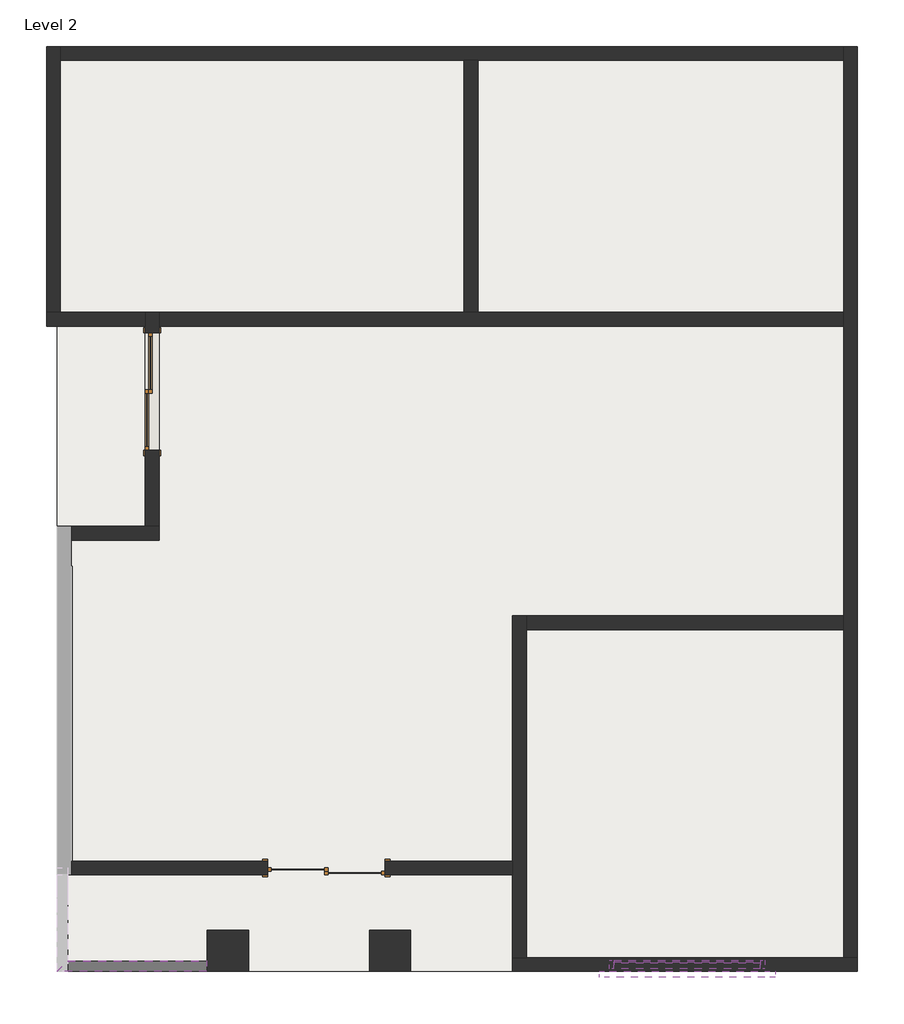
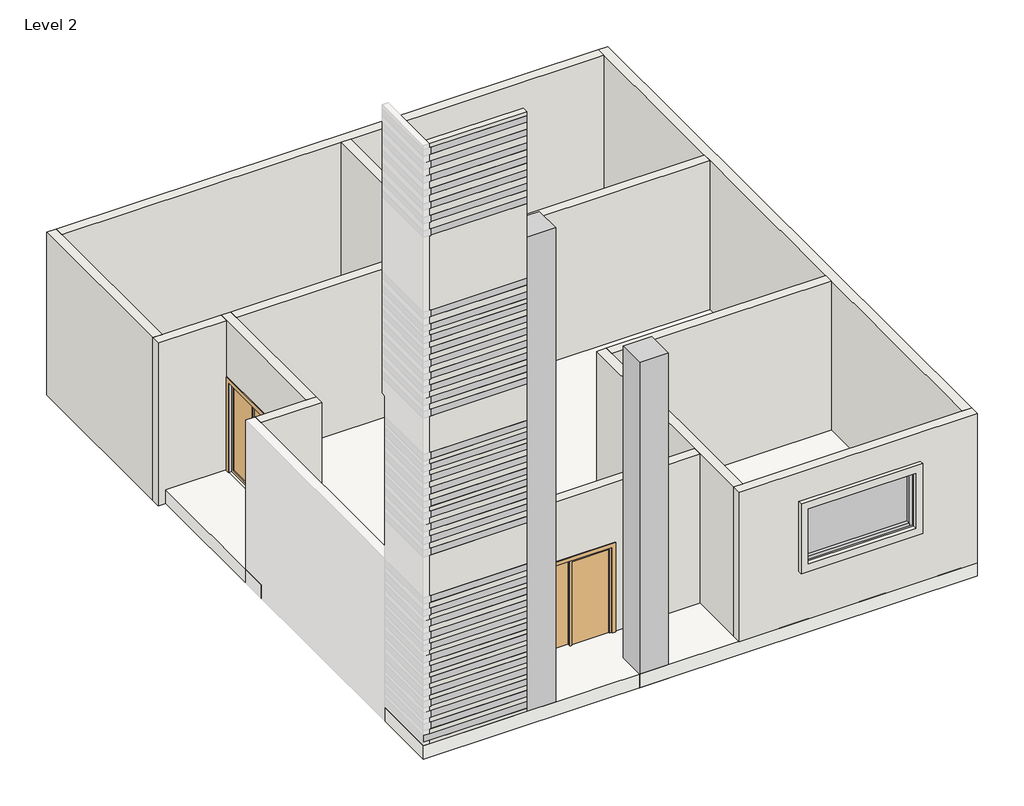
# One storey, part 2 of 2: 38 proxies, 14 walls, 8 members, 2 columns, 2 doors, 2 plates, 1 roof.
"""IFC4 building model written with IfcOpenShell, lengths in millimetres."""

from ifc_helpers import new_model, si_unit, frame, origin, place, context, project, spatial, polyline, outline, extrude, faceted_brep, transform, mapped, element, save
from components import column_feb29232, door_076b30e0, member_3a6679d5, member_c08f7e50, system_panel_glazed_5a0db22b, walls_1_walls_1_d8ce8ff7

model = new_model("IFC4")

# Units and contexts
model_context = context("Model", 3, world=origin())
ifc_project = project(units=[si_unit("LENGTHUNIT", "METRE", prefix="MILLI")], contexts=[model_context])

# Site, building, storey
site = spatial("IfcSite", under=ifc_project)
building = spatial("IfcBuilding", under=site)
storey = spatial("IfcBuildingStorey", under=building, Name="Level 2", Elevation=3657.6)

# Proxies
placement = place(None, origin())
element("IfcBuildingElementProxy", 1, Name="Reveal", ObjectType="Reveal", at=placement, inside=storey, context=model_context, shape_type="SweptSolid", body=[
    extrude(outline(polyline([(-8860.5727738, -3989.2325754), (-8708.1727738, -3836.8325754), (-6663.4727738, -3836.8325754), (-6663.4727738, -3989.2325754), (-8860.5727738, -3989.2325754)])), frame((0.0, 0.0, 4038.6), z_axis=(0.0, 0.0, 1.0), x_axis=(1.0, 0.0, 0.0)), (0.0, 0.0, 1.0), 152.4),
])
element("IfcBuildingElementProxy", 2, Name="Reveal", ObjectType="Reveal", at=placement, inside=storey, context=model_context, shape_type="SweptSolid", body=[
    extrude(outline(polyline([(-8860.5727738, -3989.2325754), (-8708.1727738, -3836.8325754), (-6663.4727738, -3836.8325754), (-6663.4727738, -3989.2325754), (-8860.5727738, -3989.2325754)])), frame((0.0, 0.0, 4292.6), z_axis=(0.0, 0.0, 1.0), x_axis=(1.0, 0.0, 0.0)), (0.0, 0.0, 1.0), 152.4),
])
element("IfcBuildingElementProxy", 3, Name="Reveal", ObjectType="Reveal", at=placement, inside=storey, context=model_context, shape_type="SweptSolid", body=[
    extrude(outline(polyline([(-8860.5727738, -3989.2325754), (-8708.1727738, -3836.8325754), (-6663.4727738, -3836.8325754), (-6663.4727738, -3989.2325754), (-8860.5727738, -3989.2325754)])), frame((0.0, 0.0, 4546.6), z_axis=(0.0, 0.0, 1.0), x_axis=(1.0, 0.0, 0.0)), (0.0, 0.0, 1.0), 152.4),
])
element("IfcBuildingElementProxy", 4, Name="Reveal", ObjectType="Reveal", at=placement, inside=storey, context=model_context, shape_type="SweptSolid", body=[
    extrude(outline(polyline([(-8860.5727738, -3989.2325754), (-8708.1727738, -3836.8325754), (-6663.4727738, -3836.8325754), (-6663.4727738, -3989.2325754), (-8860.5727738, -3989.2325754)])), frame((0.0, 0.0, 4800.6), z_axis=(0.0, 0.0, 1.0), x_axis=(1.0, 0.0, 0.0)), (0.0, 0.0, 1.0), 152.4),
])
element("IfcBuildingElementProxy", 5, Name="Reveal", ObjectType="Reveal", at=placement, inside=storey, context=model_context, shape_type="SweptSolid", body=[
    extrude(outline(polyline([(-8860.5727738, -3989.2325754), (-8708.1727738, -3836.8325754), (-6663.4727738, -3836.8325754), (-6663.4727738, -3989.2325754), (-8860.5727738, -3989.2325754)])), frame((0.0, 0.0, 5054.6), z_axis=(0.0, 0.0, 1.0), x_axis=(1.0, 0.0, 0.0)), (0.0, 0.0, 1.0), 152.4),
])
element("IfcBuildingElementProxy", 6, Name="Reveal", ObjectType="Reveal", at=placement, inside=storey, context=model_context, shape_type="SweptSolid", body=[
    extrude(outline(polyline([(-8860.5727738, -3989.2325754), (-8708.1727738, -3836.8325754), (-6663.4727738, -3836.8325754), (-6663.4727738, -3989.2325754), (-8860.5727738, -3989.2325754)])), frame((0.0, 0.0, 5308.6), z_axis=(0.0, 0.0, 1.0), x_axis=(1.0, 0.0, 0.0)), (0.0, 0.0, 1.0), 152.4),
])
element("IfcBuildingElementProxy", 7, Name="Reveal", ObjectType="Reveal", at=placement, inside=storey, context=model_context, shape_type="SweptSolid", body=[
    extrude(outline(polyline([(-8860.5727738, -3989.2325754), (-8708.1727738, -3836.8325754), (-6663.4727738, -3836.8325754), (-6663.4727738, -3989.2325754), (-8860.5727738, -3989.2325754)])), frame((0.0, 0.0, 5562.6), z_axis=(0.0, 0.0, 1.0), x_axis=(1.0, 0.0, 0.0)), (0.0, 0.0, 1.0), 152.4),
])
element("IfcBuildingElementProxy", 8, Name="Reveal", ObjectType="Reveal", at=placement, inside=storey, context=model_context, shape_type="SweptSolid", body=[
    extrude(outline(polyline([(-8860.5727738, -3989.2325754), (-8708.1727738, -3836.8325754), (-6663.4727738, -3836.8325754), (-6663.4727738, -3989.2325754), (-8860.5727738, -3989.2325754)])), frame((0.0, 0.0, 5816.6), z_axis=(0.0, 0.0, 1.0), x_axis=(1.0, 0.0, 0.0)), (0.0, 0.0, 1.0), 152.4),
])
element("IfcBuildingElementProxy", 9, Name="Reveal", ObjectType="Reveal", at=placement, inside=storey, context=model_context, shape_type="SweptSolid", body=[
    extrude(outline(polyline([(-8860.5727738, -3989.2325754), (-8708.1727738, -3836.8325754), (-6663.4727738, -3836.8325754), (-6663.4727738, -3989.2325754), (-8860.5727738, -3989.2325754)])), frame((0.0, 0.0, 6070.6), z_axis=(0.0, 0.0, 1.0), x_axis=(1.0, 0.0, 0.0)), (0.0, 0.0, 1.0), 152.4),
])
element("IfcBuildingElementProxy", 10, Name="Reveal", ObjectType="Reveal", at=placement, inside=storey, context=model_context, shape_type="SweptSolid", body=[
    extrude(outline(polyline([(-8860.5727738, -3989.2325754), (-8708.1727738, -3836.8325754), (-6663.4727738, -3836.8325754), (-6663.4727738, -3989.2325754), (-8860.5727738, -3989.2325754)])), frame((0.0, 0.0, 6324.6), z_axis=(0.0, 0.0, 1.0), x_axis=(1.0, 0.0, 0.0)), (0.0, 0.0, 1.0), 152.4),
])
element("IfcBuildingElementProxy", 11, Name="Reveal", ObjectType="Reveal", at=placement, inside=storey, context=model_context, shape_type="SweptSolid", body=[
    extrude(outline(polyline([(-8860.5727738, -3989.2325754), (-8708.1727738, -3836.8325754), (-6663.4727738, -3836.8325754), (-6663.4727738, -3989.2325754), (-8860.5727738, -3989.2325754)])), frame((0.0, 0.0, 6604.0), z_axis=(0.0, 0.0, 1.0), x_axis=(1.0, 0.0, 0.0)), (0.0, 0.0, 1.0), 152.4),
])
element("IfcBuildingElementProxy", 12, Name="Reveal", ObjectType="Reveal", at=placement, inside=storey, context=model_context, shape_type="SweptSolid", body=[
    extrude(outline(polyline([(-8860.5727738, -3989.2325754), (-8708.1727738, -3836.8325754), (-6663.4727738, -3836.8325754), (-6663.4727738, -3989.2325754), (-8860.5727738, -3989.2325754)])), frame((0.0, 0.0, 6858.0), z_axis=(0.0, 0.0, 1.0), x_axis=(1.0, 0.0, 0.0)), (0.0, 0.0, 1.0), 152.4),
])
element("IfcBuildingElementProxy", 13, Name="Reveal", ObjectType="Reveal", at=placement, inside=storey, context=model_context, shape_type="SweptSolid", body=[
    extrude(outline(polyline([(-8860.5727738, -3989.2325754), (-8708.1727738, -3836.8325754), (-6663.4727738, -3836.8325754), (-6663.4727738, -3989.2325754), (-8860.5727738, -3989.2325754)])), frame((0.0, 0.0, 7137.4), z_axis=(0.0, 0.0, 1.0), x_axis=(1.0, 0.0, 0.0)), (0.0, 0.0, 1.0), 152.4),
])
element("IfcBuildingElementProxy", 14, Name="Reveal", ObjectType="Reveal", at=placement, inside=storey, context=model_context, shape_type="SweptSolid", body=[
    extrude(outline(polyline([(-8860.5727738, -3989.2325754), (-8708.1727738, -3836.8325754), (-6663.4727738, -3836.8325754), (-6663.4727738, -3989.2325754), (-8860.5727738, -3989.2325754)])), frame((0.0, 0.0, 8204.2), z_axis=(0.0, 0.0, 1.0), x_axis=(1.0, 0.0, 0.0)), (0.0, 0.0, 1.0), 152.4),
])
element("IfcBuildingElementProxy", 15, Name="Reveal", ObjectType="Reveal", at=placement, inside=storey, context=model_context, shape_type="SweptSolid", body=[
    extrude(outline(polyline([(-8860.5727738, -3989.2325754), (-8708.1727738, -3836.8325754), (-6663.4727738, -3836.8325754), (-6663.4727738, -3989.2325754), (-8860.5727738, -3989.2325754)])), frame((0.0, 0.0, 8483.6), z_axis=(0.0, 0.0, 1.0), x_axis=(1.0, 0.0, 0.0)), (0.0, 0.0, 1.0), 152.4),
])
element("IfcBuildingElementProxy", 16, Name="Reveal", ObjectType="Reveal", at=placement, inside=storey, context=model_context, shape_type="SweptSolid", body=[
    extrude(outline(polyline([(-8860.5727738, -3989.2325754), (-8708.1727738, -3836.8325754), (-6663.4727738, -3836.8325754), (-6663.4727738, -3989.2325754), (-8860.5727738, -3989.2325754)])), frame((0.0, 0.0, 8763.0), z_axis=(0.0, 0.0, 1.0), x_axis=(1.0, 0.0, 0.0)), (0.0, 0.0, 1.0), 152.4),
])
element("IfcBuildingElementProxy", 17, Name="Reveal", ObjectType="Reveal", at=placement, inside=storey, context=model_context, shape_type="SweptSolid", body=[
    extrude(outline(polyline([(-8860.5727738, -3989.2325754), (-8708.1727738, -3836.8325754), (-6663.4727738, -3836.8325754), (-6663.4727738, -3989.2325754), (-8860.5727738, -3989.2325754)])), frame((0.0, 0.0, 9042.4), z_axis=(0.0, 0.0, 1.0), x_axis=(1.0, 0.0, 0.0)), (0.0, 0.0, 1.0), 152.4),
])
element("IfcBuildingElementProxy", 18, Name="Reveal", ObjectType="Reveal", at=placement, inside=storey, context=model_context, shape_type="SweptSolid", body=[
    extrude(outline(polyline([(-8860.5727738, -3989.2325754), (-8708.1727738, -3836.8325754), (-6663.4727738, -3836.8325754), (-6663.4727738, -3989.2325754), (-8860.5727738, -3989.2325754)])), frame((0.0, 0.0, 9296.4), z_axis=(0.0, 0.0, 1.0), x_axis=(1.0, 0.0, 0.0)), (0.0, 0.0, 1.0), 152.4),
])
element("IfcBuildingElementProxy", 19, Name="Reveal", ObjectType="Reveal", at=placement, inside=storey, context=model_context, shape_type="SweptSolid", body=[
    extrude(outline(polyline([(-8860.5727738, -3989.2325754), (-8708.1727738, -3836.8325754), (-6663.4727738, -3836.8325754), (-6663.4727738, -3989.2325754), (-8860.5727738, -3989.2325754)])), frame((0.0, 0.0, 9575.8), z_axis=(0.0, 0.0, 1.0), x_axis=(1.0, 0.0, 0.0)), (0.0, 0.0, 1.0), 152.4),
])
element("IfcBuildingElementProxy", 20, Name="Reveal", ObjectType="Reveal", at=placement, inside=storey, context=model_context, shape_type="SweptSolid", body=[
    extrude(outline(polyline([(-8860.5727738, -3989.2325754), (-8708.1727738, -3836.8325754), (-6663.4727738, -3836.8325754), (-6663.4727738, -3989.2325754), (-8860.5727738, -3989.2325754)])), frame((0.0, 0.0, 9855.2), z_axis=(0.0, 0.0, 1.0), x_axis=(1.0, 0.0, 0.0)), (0.0, 0.0, 1.0), 152.4),
])
element("IfcBuildingElementProxy", 21, Name="Reveal", ObjectType="Reveal", at=placement, inside=storey, context=model_context, shape_type="SweptSolid", body=[
    extrude(outline(polyline([(-8860.5727738, -3989.2325754), (-8708.1727738, -3836.8325754), (-6663.4727738, -3836.8325754), (-6663.4727738, -3989.2325754), (-8860.5727738, -3989.2325754)])), frame((0.0, 0.0, 10109.2), z_axis=(0.0, 0.0, 1.0), x_axis=(1.0, 0.0, 0.0)), (0.0, 0.0, 1.0), 152.4),
])
element("IfcBuildingElementProxy", 22, Name="Reveal", ObjectType="Reveal", at=placement, inside=storey, context=model_context, shape_type="SweptSolid", body=[
    extrude(outline(polyline([(-8860.5727738, -3989.2325754), (-8708.1727738, -3836.8325754), (-6663.4727738, -3836.8325754), (-6663.4727738, -3989.2325754), (-8860.5727738, -3989.2325754)])), frame((0.0, 0.0, 10363.2), z_axis=(0.0, 0.0, 1.0), x_axis=(1.0, 0.0, 0.0)), (0.0, 0.0, 1.0), 152.4),
])
element("IfcBuildingElementProxy", 23, Name="Reveal", ObjectType="Reveal", at=placement, inside=storey, context=model_context, shape_type="SweptSolid", body=[
    extrude(outline(polyline([(-8860.5727738, -3989.2325754), (-8708.1727738, -3836.8325754), (-6663.4727738, -3836.8325754), (-6663.4727738, -3989.2325754), (-8860.5727738, -3989.2325754)])), frame((0.0, 0.0, 11328.4), z_axis=(0.0, 0.0, 1.0), x_axis=(1.0, 0.0, 0.0)), (0.0, 0.0, 1.0), 152.4),
])
element("IfcBuildingElementProxy", 24, Name="Reveal", ObjectType="Reveal", at=placement, inside=storey, context=model_context, shape_type="SweptSolid", body=[
    extrude(outline(polyline([(-8860.5727738, -3989.2325754), (-8708.1727738, -3836.8325754), (-6663.4727738, -3836.8325754), (-6663.4727738, -3989.2325754), (-8860.5727738, -3989.2325754)])), frame((0.0, 0.0, 11607.8), z_axis=(0.0, 0.0, 1.0), x_axis=(1.0, 0.0, 0.0)), (0.0, 0.0, 1.0), 152.4),
])
element("IfcBuildingElementProxy", 25, Name="Reveal", ObjectType="Reveal", at=placement, inside=storey, context=model_context, shape_type="SweptSolid", body=[
    extrude(outline(polyline([(-8860.5727738, -3989.2325754), (-8708.1727738, -3836.8325754), (-6663.4727738, -3836.8325754), (-6663.4727738, -3989.2325754), (-8860.5727738, -3989.2325754)])), frame((0.0, 0.0, 11887.2), z_axis=(0.0, 0.0, 1.0), x_axis=(1.0, 0.0, 0.0)), (0.0, 0.0, 1.0), 152.4),
])
element("IfcBuildingElementProxy", 26, Name="Reveal", ObjectType="Reveal", at=placement, inside=storey, context=model_context, shape_type="SweptSolid", body=[
    extrude(outline(polyline([(-8860.5727738, -3989.2325754), (-8708.1727738, -3836.8325754), (-6663.4727738, -3836.8325754), (-6663.4727738, -3989.2325754), (-8860.5727738, -3989.2325754)])), frame((0.0, 0.0, 12166.6), z_axis=(0.0, 0.0, 1.0), x_axis=(1.0, 0.0, 0.0)), (0.0, 0.0, 1.0), 152.4),
])
element("IfcBuildingElementProxy", 27, Name="Reveal", ObjectType="Reveal", at=placement, inside=storey, context=model_context, shape_type="SweptSolid", body=[
    extrude(outline(polyline([(-8860.5727738, -3989.2325754), (-8708.1727738, -3836.8325754), (-6663.4727738, -3836.8325754), (-6663.4727738, -3989.2325754), (-8860.5727738, -3989.2325754)])), frame((0.0, 0.0, 12446.0), z_axis=(0.0, 0.0, 1.0), x_axis=(1.0, 0.0, 0.0)), (0.0, 0.0, 1.0), 152.4),
])
element("IfcBuildingElementProxy", 28, Name="Reveal", ObjectType="Reveal", at=placement, inside=storey, context=model_context, shape_type="SweptSolid", body=[
    extrude(outline(polyline([(-8860.5727738, -3989.2325754), (-8708.1727738, -3836.8325754), (-6663.4727738, -3836.8325754), (-6663.4727738, -3989.2325754), (-8860.5727738, -3989.2325754)])), frame((0.0, 0.0, 12725.4), z_axis=(0.0, 0.0, 1.0), x_axis=(1.0, 0.0, 0.0)), (0.0, 0.0, 1.0), 152.4),
])
element("IfcBuildingElementProxy", 29, Name="Reveal", ObjectType="Reveal", at=placement, inside=storey, context=model_context, shape_type="SweptSolid", body=[
    extrude(outline(polyline([(-8860.5727738, -3989.2325754), (-8708.1727738, -3836.8325754), (-6663.4727738, -3836.8325754), (-6663.4727738, -3989.2325754), (-8860.5727738, -3989.2325754)])), frame((0.0, 0.0, 13004.8), z_axis=(0.0, 0.0, 1.0), x_axis=(1.0, 0.0, 0.0)), (0.0, 0.0, 1.0), 152.4),
])
element("IfcBuildingElementProxy", 30, Name="Reveal", ObjectType="Reveal", at=placement, inside=storey, context=model_context, shape_type="SweptSolid", body=[
    extrude(outline(polyline([(-8860.5727738, -3989.2325754), (-8708.1727738, -3836.8325754), (-6663.4727738, -3836.8325754), (-6663.4727738, -3989.2325754), (-8860.5727738, -3989.2325754)])), frame((0.0, 0.0, 13258.8), z_axis=(0.0, 0.0, 1.0), x_axis=(1.0, 0.0, 0.0)), (0.0, 0.0, 1.0), 152.4),
])
element("IfcBuildingElementProxy", 31, Name="Reveal", ObjectType="Reveal", at=placement, inside=storey, context=model_context, shape_type="SweptSolid", body=[
    extrude(outline(polyline([(-8860.5727738, -3989.2325754), (-8708.1727738, -3836.8325754), (-6663.4727738, -3836.8325754), (-6663.4727738, -3989.2325754), (-8860.5727738, -3989.2325754)])), frame((0.0, 0.0, 13563.6), z_axis=(0.0, 0.0, 1.0), x_axis=(1.0, 0.0, 0.0)), (0.0, 0.0, 1.0), 152.4),
])
element("IfcBuildingElementProxy", 32, Name="Reveal", ObjectType="Reveal", at=placement, inside=storey, context=model_context, shape_type="SweptSolid", body=[
    extrude(outline(polyline([(-8860.5727738, -3989.2325754), (-8708.1727738, -3836.8325754), (-6663.4727738, -3836.8325754), (-6663.4727738, -3989.2325754), (-8860.5727738, -3989.2325754)])), frame((0.0, 0.0, 15392.4), z_axis=(0.0, 0.0, 1.0), x_axis=(1.0, 0.0, 0.0)), (0.0, 0.0, 1.0), 152.4),
])
element("IfcBuildingElementProxy", 33, Name="Reveal", ObjectType="Reveal", at=placement, inside=storey, context=model_context, shape_type="SweptSolid", body=[
    extrude(outline(polyline([(-8860.5727738, -3989.2325754), (-8708.1727738, -3836.8325754), (-6663.4727738, -3836.8325754), (-6663.4727738, -3989.2325754), (-8860.5727738, -3989.2325754)])), frame((0.0, 0.0, 15697.2), z_axis=(0.0, 0.0, 1.0), x_axis=(1.0, 0.0, 0.0)), (0.0, 0.0, 1.0), 152.4),
])
element("IfcBuildingElementProxy", 34, Name="Reveal", ObjectType="Reveal", at=placement, inside=storey, context=model_context, shape_type="SweptSolid", body=[
    extrude(outline(polyline([(-8860.5727738, -3989.2325754), (-8708.1727738, -3836.8325754), (-6663.4727738, -3836.8325754), (-6663.4727738, -3989.2325754), (-8860.5727738, -3989.2325754)])), frame((0.0, 0.0, 16002.0), z_axis=(0.0, 0.0, 1.0), x_axis=(1.0, 0.0, 0.0)), (0.0, 0.0, 1.0), 152.4),
])
element("IfcBuildingElementProxy", 35, Name="Reveal", ObjectType="Reveal", at=placement, inside=storey, context=model_context, shape_type="SweptSolid", body=[
    extrude(outline(polyline([(-8860.5727738, -3989.2325754), (-8708.1727738, -3836.8325754), (-6663.4727738, -3836.8325754), (-6663.4727738, -3989.2325754), (-8860.5727738, -3989.2325754)])), frame((0.0, 0.0, 16306.8), z_axis=(0.0, 0.0, 1.0), x_axis=(1.0, 0.0, 0.0)), (0.0, 0.0, 1.0), 152.4),
])
element("IfcBuildingElementProxy", 36, Name="Reveal", ObjectType="Reveal", at=placement, inside=storey, context=model_context, shape_type="SweptSolid", body=[
    extrude(outline(polyline([(-8860.5727738, -3989.2325754), (-8708.1727738, -3836.8325754), (-6663.4727738, -3836.8325754), (-6663.4727738, -3989.2325754), (-8860.5727738, -3989.2325754)])), frame((0.0, 0.0, 16611.6), z_axis=(0.0, 0.0, 1.0), x_axis=(1.0, 0.0, 0.0)), (0.0, 0.0, 1.0), 152.4),
])
element("IfcBuildingElementProxy", 37, Name="Reveal", ObjectType="Reveal", at=placement, inside=storey, context=model_context, shape_type="SweptSolid", body=[
    extrude(outline(polyline([(-8860.5727738, -3989.2325754), (-8708.1727738, -3836.8325754), (-6663.4727738, -3836.8325754), (-6663.4727738, -3989.2325754), (-8860.5727738, -3989.2325754)])), frame((0.0, 0.0, 16916.4), z_axis=(0.0, 0.0, 1.0), x_axis=(1.0, 0.0, 0.0)), (0.0, 0.0, 1.0), 152.4),
])
element("IfcBuildingElementProxy", 38, Name="Reveal", ObjectType="Reveal", at=placement, inside=storey, context=model_context, shape_type="SweptSolid", body=[
    extrude(outline(polyline([(-8860.5727738, -3989.2325754), (-8708.1727738, -3836.8325754), (-6663.4727738, -3836.8325754), (-6663.4727738, -3989.2325754), (-8860.5727738, -3989.2325754)])), frame((0.0, 0.0, 17221.2), z_axis=(0.0, 0.0, 1.0), x_axis=(1.0, 0.0, 0.0)), (0.0, 0.0, 1.0), 152.4),
])

# Columns
element("IfcColumn", 39, ObjectType="Rectangular Column : 24\" x 24\"", at=placement, inside=storey, context=model_context, shape_type="SweptSolid", body=[
    extrude(outline(polyline([(-6041.5436544, -3379.6325754), (-6041.5436544, -3989.2325754), (-6651.1436544, -3989.2325754), (-6651.1436544, -3379.6325754), (-6041.5436544, -3379.6325754)])), frame((0.0, 0.0, 3657.6), z_axis=(0.0, 0.0, 1.0), x_axis=(1.0, 0.0, 0.0)), (0.0, 0.0, 1.0), 10972.8),
])
column_shape = column_feb29232(model_context)
element("IfcColumn", 40, ObjectType="Rectangular Column : 24\" x 24\"", at=placement, inside=storey, context=model_context, shape_type="MappedRepresentation", body=[
    mapped(column_shape, transform((-3958.7436544, -3684.4325754, 0.0), x_axis=(1.0, 0.0, 0.0), y_axis=(0.0, 1.0, 0.0), z_axis=(0.0, 0.0, 1.0))),
])

# Doors
door_shape = door_076b30e0(model_context)
element("IfcDoor", 41, ObjectType="Door-Double-Sliding : 68\" x 80\"", at=placement, inside=storey, context=model_context, shape_type="MappedRepresentation", body=[
    mapped(door_shape, transform((-7336.5727738, 4545.1674246, 3962.4), x_axis=(0.0, 1.0, 0.0), y_axis=(-1.0, 0.0, 0.0), z_axis=(0.0, 0.0, 1.0))),
])
element("IfcDoor", 42, ObjectType="Door-Double-Sliding : 68\" x 80\"", at=placement, inside=storey, context=model_context, shape_type="MappedRepresentation", body=[
    mapped(door_shape, transform((-4898.5436544, -2338.2325754, 3860.8), x_axis=(-1.0, 0.0, 0.0), y_axis=(0.0, -1.0, 0.0), z_axis=(0.0, 0.0, 1.0))),
])

# Members
member_shape = member_3a6679d5(model_context)
element("IfcMember", 43, ObjectType="Rectangular Mullion : 2.5\" x 5\" rectangular", at=placement, inside=storey, context=model_context, shape_type="MappedRepresentation", body=[
    mapped(member_shape, transform((1560.0533085, -3887.6325754, 5261.1422066), x_axis=(1.0, 0.0, 0.0), y_axis=(0.0, -1.0, 0.0), z_axis=(0.0, 0.0, -1.0))),
])
element("IfcMember", 44, ObjectType="Rectangular Mullion : 2.5\" x 5\" rectangular", at=placement, inside=storey, context=model_context, shape_type="MappedRepresentation", body=[
    mapped(member_shape, transform((1560.0533085, -3887.6325754, 5261.1422066), x_axis=(1.0, 0.0, 0.0), y_axis=(0.0, -1.0, 0.0), z_axis=(0.0, 0.0, -1.0))),
])
member_2_shape = member_c08f7e50(model_context)
element("IfcMember", 45, ObjectType="Rectangular Mullion : 2.5\" x 5\" rectangular", at=placement, inside=storey, context=model_context, shape_type="MappedRepresentation", body=[
    mapped(member_2_shape, transform((-662.4466915, -3887.6325754, 5261.1422066), x_axis=(0.0, 0.0, -1.0), y_axis=(0.0, -1.0, 0.0), z_axis=(-1.0, 0.0, 0.0))),
])
element("IfcMember", 46, ObjectType="Rectangular Mullion : 2.5\" x 5\" rectangular", at=placement, inside=storey, context=model_context, shape_type="MappedRepresentation", body=[
    mapped(member_2_shape, transform((-662.4466915, -3887.6325754, 5261.1422066), x_axis=(0.0, 0.0, -1.0), y_axis=(0.0, -1.0, 0.0), z_axis=(-1.0, 0.0, 0.0))),
])
element("IfcMember", 47, ObjectType="Rectangular Mullion : 2.5\" x 5\" rectangular", at=placement, inside=storey, context=model_context, shape_type="MappedRepresentation", body=[
    mapped(member_2_shape, transform((1496.5533085, -3887.6325754, 6492.024337), x_axis=(0.0, 0.0, 1.0), y_axis=(0.0, -1.0, 0.0), z_axis=(1.0, 0.0, 0.0))),
])
element("IfcMember", 48, ObjectType="Rectangular Mullion : 2.5\" x 5\" rectangular", at=placement, inside=storey, context=model_context, shape_type="MappedRepresentation", body=[
    mapped(member_2_shape, transform((1496.5533085, -3887.6325754, 6492.024337), x_axis=(0.0, 0.0, 1.0), y_axis=(0.0, -1.0, 0.0), z_axis=(1.0, 0.0, 0.0))),
])
element("IfcMember", 49, ObjectType="Rectangular Mullion : 2.5\" x 5\" rectangular", at=placement, inside=storey, context=model_context, shape_type="MappedRepresentation", body=[
    mapped(member_shape, transform((-725.9466915, -3887.6325754, 6492.024337), x_axis=(-1.0, 0.0, 0.0), y_axis=(0.0, -1.0, 0.0), z_axis=(0.0, 0.0, 1.0))),
])
element("IfcMember", 50, ObjectType="Rectangular Mullion : 2.5\" x 5\" rectangular", at=placement, inside=storey, context=model_context, shape_type="MappedRepresentation", body=[
    mapped(member_shape, transform((-725.9466915, -3887.6325754, 6492.024337), x_axis=(-1.0, 0.0, 0.0), y_axis=(0.0, -1.0, 0.0), z_axis=(0.0, 0.0, 1.0))),
])

# Plates
system_panel_glazed_shape = system_panel_glazed_5a0db22b(model_context)
element("IfcPlate", 51, ObjectType="System Panel : Glazed", at=placement, inside=storey, context=model_context, shape_type="MappedRepresentation", body=[
    mapped(system_panel_glazed_shape, transform((417.0533085, -3887.6325754, 5324.6422066), x_axis=(1.0, 0.0, 0.0), y_axis=(0.0, 1.0, 0.0), z_axis=(0.0, 0.0, 1.0))),
])
element("IfcPlate", 52, ObjectType="System Panel : Glazed", at=placement, inside=storey, context=model_context, shape_type="MappedRepresentation", body=[
    mapped(system_panel_glazed_shape, transform((417.0533085, -3887.6325754, 5324.6422066), x_axis=(1.0, 0.0, 0.0), y_axis=(0.0, 1.0, 0.0), z_axis=(0.0, 0.0, 1.0))),
])

# Roof
element("IfcRoof", 53, ObjectType="Generic - 12\"", at=placement, inside=storey, context=model_context, shape_type="SweptSolid", body=[
    extrude(outline(polyline([(-8860.5727738, 9472.7674246), (2924.6563456, 9472.7674246), (2924.6563456, -3989.2325754), (-8860.5727738, -3989.2325754), (-8860.5727738, -2566.8325754), (-8631.9727738, -2566.8325754), (-8631.9727738, 1979.7674246), (-8860.5727738, 1979.7674246), (-8860.5727738, 9472.7674246)])), frame((0.0, 0.0, 3657.6), z_axis=(0.0, 0.0, 1.0), x_axis=(1.0, 0.0, 0.0)), (0.0, 0.0, 1.0), 304.8),
])

# Walls
element("IfcWall", 54, ObjectType="Generic - 5\"", at=placement, inside=storey, context=model_context, shape_type="SweptSolid", body=[
    extrude(outline(polyline([(-6663.4727738, -3989.2325754), (-8733.5727738, -3989.2325754), (-8733.5727738, -3862.2325754), (-6663.4727738, -3862.2325754), (-6663.4727738, -3989.2325754)])), frame((0.0, 0.0, 3962.4), z_axis=(0.0, 0.0, 1.0), x_axis=(1.0, 0.0, 0.0)), (0.0, 0.0, 1.0), 76.2),
    extrude(outline(polyline([(-8733.5727738, -3989.2325754), (-8733.5727738, -3862.2325754), (-6663.4727738, -3862.2325754), (-6663.4727738, -3989.2325754), (-8733.5727738, -3989.2325754)])), frame((0.0, 0.0, 17373.6), z_axis=(0.0, 0.0, 1.0), x_axis=(1.0, 0.0, 0.0)), (0.0, 0.0, 1.0), 91.224337),
    extrude(outline(polyline([(-8733.5727738, -3989.2325754), (-8733.5727738, -3862.2325754), (-6663.4727738, -3862.2325754), (-6663.4727738, -3989.2325754), (-8733.5727738, -3989.2325754)])), frame((0.0, 0.0, 4445.0), z_axis=(0.0, 0.0, 1.0), x_axis=(1.0, 0.0, 0.0)), (0.0, 0.0, 1.0), 101.6),
    extrude(outline(polyline([(-6663.4727738, -3989.2325754), (-8733.5727738, -3989.2325754), (-8733.5727738, -3862.2325754), (-6663.4727738, -3862.2325754), (-6663.4727738, -3989.2325754)])), frame((0.0, 0.0, 4191.0), z_axis=(0.0, 0.0, 1.0), x_axis=(1.0, 0.0, 0.0)), (0.0, 0.0, 1.0), 101.6),
    extrude(outline(polyline([(-8733.5727738, -3989.2325754), (-8733.5727738, -3862.2325754), (-6663.4727738, -3862.2325754), (-6663.4727738, -3989.2325754), (-8733.5727738, -3989.2325754)])), frame((0.0, 0.0, 4699.0), z_axis=(0.0, 0.0, 1.0), x_axis=(1.0, 0.0, 0.0)), (0.0, 0.0, 1.0), 101.6),
    extrude(outline(polyline([(-8733.5727738, -3989.2325754), (-8733.5727738, -3862.2325754), (-6663.4727738, -3862.2325754), (-6663.4727738, -3989.2325754), (-8733.5727738, -3989.2325754)])), frame((0.0, 0.0, 4953.0), z_axis=(0.0, 0.0, 1.0), x_axis=(1.0, 0.0, 0.0)), (0.0, 0.0, 1.0), 101.6),
    extrude(outline(polyline([(-8733.5727738, -3989.2325754), (-8733.5727738, -3862.2325754), (-6663.4727738, -3862.2325754), (-6663.4727738, -3989.2325754), (-8733.5727738, -3989.2325754)])), frame((0.0, 0.0, 5207.0), z_axis=(0.0, 0.0, 1.0), x_axis=(1.0, 0.0, 0.0)), (0.0, 0.0, 1.0), 101.6),
    extrude(outline(polyline([(-8733.5727738, -3989.2325754), (-8733.5727738, -3862.2325754), (-6663.4727738, -3862.2325754), (-6663.4727738, -3989.2325754), (-8733.5727738, -3989.2325754)])), frame((0.0, 0.0, 5461.0), z_axis=(0.0, 0.0, 1.0), x_axis=(1.0, 0.0, 0.0)), (0.0, 0.0, 1.0), 101.6),
    extrude(outline(polyline([(-8733.5727738, -3989.2325754), (-8733.5727738, -3862.2325754), (-6663.4727738, -3862.2325754), (-6663.4727738, -3989.2325754), (-8733.5727738, -3989.2325754)])), frame((0.0, 0.0, 5715.0), z_axis=(0.0, 0.0, 1.0), x_axis=(1.0, 0.0, 0.0)), (0.0, 0.0, 1.0), 101.6),
    extrude(outline(polyline([(-8733.5727738, -3989.2325754), (-8733.5727738, -3862.2325754), (-6663.4727738, -3862.2325754), (-6663.4727738, -3989.2325754), (-8733.5727738, -3989.2325754)])), frame((0.0, 0.0, 5969.0), z_axis=(0.0, 0.0, 1.0), x_axis=(1.0, 0.0, 0.0)), (0.0, 0.0, 1.0), 101.6),
    extrude(outline(polyline([(-8733.5727738, -3989.2325754), (-8733.5727738, -3862.2325754), (-6663.4727738, -3862.2325754), (-6663.4727738, -3989.2325754), (-8733.5727738, -3989.2325754)])), frame((0.0, 0.0, 6223.0), z_axis=(0.0, 0.0, 1.0), x_axis=(1.0, 0.0, 0.0)), (0.0, 0.0, 1.0), 101.6),
    extrude(outline(polyline([(-8733.5727738, -3989.2325754), (-8733.5727738, -3862.2325754), (-6663.4727738, -3862.2325754), (-6663.4727738, -3989.2325754), (-8733.5727738, -3989.2325754)])), frame((0.0, 0.0, 6477.0), z_axis=(0.0, 0.0, 1.0), x_axis=(1.0, 0.0, 0.0)), (0.0, 0.0, 1.0), 127.0),
    extrude(outline(polyline([(-8733.5727738, -3989.2325754), (-8733.5727738, -3862.2325754), (-6663.4727738, -3862.2325754), (-6663.4727738, -3989.2325754), (-8733.5727738, -3989.2325754)])), frame((0.0, 0.0, 6756.4), z_axis=(0.0, 0.0, 1.0), x_axis=(1.0, 0.0, 0.0)), (0.0, 0.0, 1.0), 101.6),
    extrude(outline(polyline([(-8733.5727738, -3989.2325754), (-8733.5727738, -3862.2325754), (-6663.4727738, -3862.2325754), (-6663.4727738, -3989.2325754), (-8733.5727738, -3989.2325754)])), frame((0.0, 0.0, 7010.4), z_axis=(0.0, 0.0, 1.0), x_axis=(1.0, 0.0, 0.0)), (0.0, 0.0, 1.0), 127.0),
    extrude(outline(polyline([(-8733.5727738, -3989.2325754), (-8733.5727738, -3862.2325754), (-6663.4727738, -3862.2325754), (-6663.4727738, -3989.2325754), (-8733.5727738, -3989.2325754)])), frame((0.0, 0.0, 7289.8), z_axis=(0.0, 0.0, 1.0), x_axis=(1.0, 0.0, 0.0)), (0.0, 0.0, 1.0), 914.4),
    extrude(outline(polyline([(-8733.5727738, -3989.2325754), (-8733.5727738, -3862.2325754), (-6663.4727738, -3862.2325754), (-6663.4727738, -3989.2325754), (-8733.5727738, -3989.2325754)])), frame((0.0, 0.0, 8356.6), z_axis=(0.0, 0.0, 1.0), x_axis=(1.0, 0.0, 0.0)), (0.0, 0.0, 1.0), 127.0),
    extrude(outline(polyline([(-8733.5727738, -3989.2325754), (-8733.5727738, -3862.2325754), (-6663.4727738, -3862.2325754), (-6663.4727738, -3989.2325754), (-8733.5727738, -3989.2325754)])), frame((0.0, 0.0, 8636.0), z_axis=(0.0, 0.0, 1.0), x_axis=(1.0, 0.0, 0.0)), (0.0, 0.0, 1.0), 127.0),
    extrude(outline(polyline([(-8733.5727738, -3989.2325754), (-8733.5727738, -3862.2325754), (-6663.4727738, -3862.2325754), (-6663.4727738, -3989.2325754), (-8733.5727738, -3989.2325754)])), frame((0.0, 0.0, 8915.4), z_axis=(0.0, 0.0, 1.0), x_axis=(1.0, 0.0, 0.0)), (0.0, 0.0, 1.0), 127.0),
    extrude(outline(polyline([(-8733.5727738, -3989.2325754), (-8733.5727738, -3862.2325754), (-6663.4727738, -3862.2325754), (-6663.4727738, -3989.2325754), (-8733.5727738, -3989.2325754)])), frame((0.0, 0.0, 9194.8), z_axis=(0.0, 0.0, 1.0), x_axis=(1.0, 0.0, 0.0)), (0.0, 0.0, 1.0), 101.6),
    extrude(outline(polyline([(-8733.5727738, -3989.2325754), (-8733.5727738, -3862.2325754), (-6663.4727738, -3862.2325754), (-6663.4727738, -3989.2325754), (-8733.5727738, -3989.2325754)])), frame((0.0, 0.0, 9448.8), z_axis=(0.0, 0.0, 1.0), x_axis=(1.0, 0.0, 0.0)), (0.0, 0.0, 1.0), 127.0),
    extrude(outline(polyline([(-8733.5727738, -3989.2325754), (-8733.5727738, -3862.2325754), (-6663.4727738, -3862.2325754), (-6663.4727738, -3989.2325754), (-8733.5727738, -3989.2325754)])), frame((0.0, 0.0, 9728.2), z_axis=(0.0, 0.0, 1.0), x_axis=(1.0, 0.0, 0.0)), (0.0, 0.0, 1.0), 127.0),
    extrude(outline(polyline([(-8733.5727738, -3989.2325754), (-8733.5727738, -3862.2325754), (-6663.4727738, -3862.2325754), (-6663.4727738, -3989.2325754), (-8733.5727738, -3989.2325754)])), frame((0.0, 0.0, 10007.6), z_axis=(0.0, 0.0, 1.0), x_axis=(1.0, 0.0, 0.0)), (0.0, 0.0, 1.0), 101.6),
    extrude(outline(polyline([(-8733.5727738, -3989.2325754), (-8733.5727738, -3862.2325754), (-6663.4727738, -3862.2325754), (-6663.4727738, -3989.2325754), (-8733.5727738, -3989.2325754)])), frame((0.0, 0.0, 10261.6), z_axis=(0.0, 0.0, 1.0), x_axis=(1.0, 0.0, 0.0)), (0.0, 0.0, 1.0), 101.6),
    extrude(outline(polyline([(-8733.5727738, -3989.2325754), (-8733.5727738, -3862.2325754), (-6663.4727738, -3862.2325754), (-6663.4727738, -3989.2325754), (-8733.5727738, -3989.2325754)])), frame((0.0, 0.0, 10515.6), z_axis=(0.0, 0.0, 1.0), x_axis=(1.0, 0.0, 0.0)), (0.0, 0.0, 1.0), 812.8),
    extrude(outline(polyline([(-8733.5727738, -3989.2325754), (-8733.5727738, -3862.2325754), (-6663.4727738, -3862.2325754), (-6663.4727738, -3989.2325754), (-8733.5727738, -3989.2325754)])), frame((0.0, 0.0, 11480.8), z_axis=(0.0, 0.0, 1.0), x_axis=(1.0, 0.0, 0.0)), (0.0, 0.0, 1.0), 127.0),
    extrude(outline(polyline([(-8733.5727738, -3989.2325754), (-8733.5727738, -3862.2325754), (-6663.4727738, -3862.2325754), (-6663.4727738, -3989.2325754), (-8733.5727738, -3989.2325754)])), frame((0.0, 0.0, 11760.2), z_axis=(0.0, 0.0, 1.0), x_axis=(1.0, 0.0, 0.0)), (0.0, 0.0, 1.0), 127.0),
    extrude(outline(polyline([(-8733.5727738, -3989.2325754), (-8733.5727738, -3862.2325754), (-6663.4727738, -3862.2325754), (-6663.4727738, -3989.2325754), (-8733.5727738, -3989.2325754)])), frame((0.0, 0.0, 12039.6), z_axis=(0.0, 0.0, 1.0), x_axis=(1.0, 0.0, 0.0)), (0.0, 0.0, 1.0), 127.0),
    extrude(outline(polyline([(-8733.5727738, -3989.2325754), (-8733.5727738, -3862.2325754), (-6663.4727738, -3862.2325754), (-6663.4727738, -3989.2325754), (-8733.5727738, -3989.2325754)])), frame((0.0, 0.0, 12319.0), z_axis=(0.0, 0.0, 1.0), x_axis=(1.0, 0.0, 0.0)), (0.0, 0.0, 1.0), 127.0),
    extrude(outline(polyline([(-8733.5727738, -3989.2325754), (-8733.5727738, -3862.2325754), (-6663.4727738, -3862.2325754), (-6663.4727738, -3989.2325754), (-8733.5727738, -3989.2325754)])), frame((0.0, 0.0, 12598.4), z_axis=(0.0, 0.0, 1.0), x_axis=(1.0, 0.0, 0.0)), (0.0, 0.0, 1.0), 127.0),
    extrude(outline(polyline([(-8733.5727738, -3989.2325754), (-8733.5727738, -3862.2325754), (-6663.4727738, -3862.2325754), (-6663.4727738, -3989.2325754), (-8733.5727738, -3989.2325754)])), frame((0.0, 0.0, 12877.8), z_axis=(0.0, 0.0, 1.0), x_axis=(1.0, 0.0, 0.0)), (0.0, 0.0, 1.0), 127.0),
    extrude(outline(polyline([(-8733.5727738, -3989.2325754), (-8733.5727738, -3862.2325754), (-6663.4727738, -3862.2325754), (-6663.4727738, -3989.2325754), (-8733.5727738, -3989.2325754)])), frame((0.0, 0.0, 13157.2), z_axis=(0.0, 0.0, 1.0), x_axis=(1.0, 0.0, 0.0)), (0.0, 0.0, 1.0), 101.6),
    extrude(outline(polyline([(-8733.5727738, -3989.2325754), (-8733.5727738, -3862.2325754), (-6663.4727738, -3862.2325754), (-6663.4727738, -3989.2325754), (-8733.5727738, -3989.2325754)])), frame((0.0, 0.0, 13411.2), z_axis=(0.0, 0.0, 1.0), x_axis=(1.0, 0.0, 0.0)), (0.0, 0.0, 1.0), 152.4),
    extrude(outline(polyline([(-8733.5727738, -3989.2325754), (-8733.5727738, -3862.2325754), (-6663.4727738, -3862.2325754), (-6663.4727738, -3989.2325754), (-8733.5727738, -3989.2325754)])), frame((0.0, 0.0, 13716.0), z_axis=(0.0, 0.0, 1.0), x_axis=(1.0, 0.0, 0.0)), (0.0, 0.0, 1.0), 1676.4),
    extrude(outline(polyline([(-8733.5727738, -3989.2325754), (-8733.5727738, -3862.2325754), (-6663.4727738, -3862.2325754), (-6663.4727738, -3989.2325754), (-8733.5727738, -3989.2325754)])), frame((0.0, 0.0, 15544.8), z_axis=(0.0, 0.0, 1.0), x_axis=(1.0, 0.0, 0.0)), (0.0, 0.0, 1.0), 152.4),
    extrude(outline(polyline([(-8733.5727738, -3989.2325754), (-8733.5727738, -3862.2325754), (-6663.4727738, -3862.2325754), (-6663.4727738, -3989.2325754), (-8733.5727738, -3989.2325754)])), frame((0.0, 0.0, 15849.6), z_axis=(0.0, 0.0, 1.0), x_axis=(1.0, 0.0, 0.0)), (0.0, 0.0, 1.0), 152.4),
    extrude(outline(polyline([(-8733.5727738, -3989.2325754), (-8733.5727738, -3862.2325754), (-6663.4727738, -3862.2325754), (-6663.4727738, -3989.2325754), (-8733.5727738, -3989.2325754)])), frame((0.0, 0.0, 16154.4), z_axis=(0.0, 0.0, 1.0), x_axis=(1.0, 0.0, 0.0)), (0.0, 0.0, 1.0), 152.4),
    extrude(outline(polyline([(-8733.5727738, -3989.2325754), (-8733.5727738, -3862.2325754), (-6663.4727738, -3862.2325754), (-6663.4727738, -3989.2325754), (-8733.5727738, -3989.2325754)])), frame((0.0, 0.0, 16459.2), z_axis=(0.0, 0.0, 1.0), x_axis=(1.0, 0.0, 0.0)), (0.0, 0.0, 1.0), 152.4),
    extrude(outline(polyline([(-8733.5727738, -3989.2325754), (-8733.5727738, -3862.2325754), (-6663.4727738, -3862.2325754), (-6663.4727738, -3989.2325754), (-8733.5727738, -3989.2325754)])), frame((0.0, 0.0, 16764.0), z_axis=(0.0, 0.0, 1.0), x_axis=(1.0, 0.0, 0.0)), (0.0, 0.0, 1.0), 152.4),
    extrude(outline(polyline([(-8733.5727738, -3989.2325754), (-8733.5727738, -3862.2325754), (-6663.4727738, -3862.2325754), (-6663.4727738, -3989.2325754), (-8733.5727738, -3989.2325754)])), frame((0.0, 0.0, 17068.8), z_axis=(0.0, 0.0, 1.0), x_axis=(1.0, 0.0, 0.0)), (0.0, 0.0, 1.0), 152.4),
])
element("IfcWall", 55, ObjectType="Generic - 8\"", at=placement, inside=storey, context=model_context, shape_type="Brep", body=[
    faceted_brep([(2924.6563456, -3786.0325754, 3950.7178696), (-2155.3436544, -3786.0325754, 3950.7178696), (-2155.3436544, -3786.0325754, 7315.2), (-1952.1436544, -3786.0325754, 7315.2), (2721.4563456, -3786.0325754, 7315.2), (2924.6563456, -3786.0325754, 7315.2), (1560.0533085, -3786.0325754, 6492.024337), (-725.9466915, -3786.0325754, 6492.024337), (-725.9466915, -3786.0325754, 5261.1422066), (1560.0533085, -3786.0325754, 5261.1422066), (2924.6563456, -3989.2325754, 3950.7178696), (2924.6563456, -3989.2325754, 7315.2), (-2155.3436544, -3989.2325754, 7315.2), (-2155.3436544, -3989.2325754, 3950.7178696), (1560.0533085, -3989.2325754, 6492.024337), (1560.0533085, -3989.2325754, 5261.1422066), (-725.9466915, -3989.2325754, 5261.1422066), (-725.9466915, -3989.2325754, 6492.024337)], [[[0, 1, 2, 3, 4, 5], [6, 7, 8, 9]], [[10, 11, 12, 13], [14, 15, 16, 17]], [[2, 1, 13, 12]], [[0, 5, 11, 10]], [[1, 0, 10, 13]], [[5, 4, 3, 2, 12, 11]], [[7, 6, 14, 17]], [[8, 7, 17, 16]], [[9, 8, 16, 15]], [[6, 9, 15, 14]]]),
])
element("IfcWall", 56, ObjectType="Generic - 8\"", at=placement, inside=storey, context=model_context, shape_type="Brep", body=[
    faceted_brep([(-1952.1436544, -3786.0325754, 3657.6), (-1952.1436544, 1039.9674246, 3657.6), (-1952.1436544, 1243.1674246, 3657.6), (-1952.1436544, 1243.1674246, 7315.2), (-1952.1436544, 1039.9674246, 7315.2), (-1952.1436544, -3786.0325754, 7315.2), (-2155.3436544, -3786.0325754, 3657.6), (-2155.3436544, -3786.0325754, 3950.7178696), (-2155.3436544, -3786.0325754, 7315.2), (-2155.3436544, -2566.8325754, 7315.2), (-2155.3436544, -2363.6325754, 7315.2), (-2155.3436544, 1243.1674246, 7315.2), (-2155.3436544, 1243.1674246, 3657.6), (-2155.3436544, -2363.6325754, 3657.6), (-2155.3436544, -2566.8325754, 3657.6)], [[[0, 1, 2, 3, 4, 5]], [[6, 7, 8, 9, 10, 11, 12, 13, 14]], [[2, 1, 0, 6, 14, 13, 12]], [[5, 4, 3, 11, 10, 9, 8]], [[0, 5, 8, 7, 6]], [[3, 2, 12, 11]]]),
])
element("IfcWall", 57, ObjectType="Generic - 8\"", at=placement, inside=storey, context=model_context, shape_type="SweptSolid", body=[
    extrude(outline(polyline([(2716.475018, 1039.9674246), (-1952.1436544, 1039.9674246), (-1952.1436544, 1243.1674246), (2716.475018, 1243.1674246), (2716.475018, 1039.9674246)])), frame((0.0, 0.0, 3657.6), z_axis=(0.0, 0.0, 1.0), x_axis=(1.0, 0.0, 0.0)), (0.0, 0.0, 1.0), 3657.6),
])
element("IfcWall", 58, ObjectType="Generic - 8\"", at=placement, inside=storey, context=model_context, shape_type="Brep", body=[
    faceted_brep([(2924.6563456, -3786.0325754, 3657.6), (2924.6563456, 9625.1674246, 3657.6), (2924.6563456, 9625.1674246, 7315.2), (2924.6563456, -3786.0325754, 7315.2), (2924.6563456, -3786.0325754, 3950.7178696), (2721.4563456, -3786.0325754, 3657.6), (2721.4563456, -3786.0325754, 7315.2), (2721.4563456, 9625.1674246, 7315.2), (2721.4563456, 9625.1674246, 3657.6)], [[[0, 1, 2, 3, 4]], [[5, 6, 7, 8]], [[1, 0, 5, 8]], [[2, 1, 8, 7]], [[3, 2, 7, 6]], [[0, 4, 3, 6, 5]]]),
])
element("IfcWall", 59, ObjectType="Generic - 8\"", at=placement, inside=storey, context=model_context, shape_type="Brep", body=[
    faceted_brep([(-8657.3727738, 2360.7674246, 3657.6), (-7361.9727738, 2360.7674246, 3657.6), (-7361.9727738, 2360.7674246, 7315.2), (-8657.3727738, 2360.7674246, 7315.2), (-8657.3727738, 2563.9674246, 3657.6), (-8657.3727738, 2563.9674246, 7315.2), (-7565.1727738, 2563.9674246, 7315.2), (-7361.9727738, 2563.9674246, 7315.2), (-7361.9727738, 2563.9674246, 3657.6), (-7565.1727738, 2563.9674246, 3657.6)], [[[0, 1, 2, 3]], [[4, 5, 6, 7, 8, 9]], [[1, 0, 4, 9, 8]], [[3, 2, 7, 6, 5]], [[0, 3, 5, 4]], [[2, 1, 8, 7]]]),
])
element("IfcWall", 60, ObjectType="Generic - 8\"", at=placement, inside=storey, context=model_context, shape_type="Brep", body=[
    faceted_brep([(-7361.9727738, 2563.9674246, 3657.6), (-7361.9727738, 5510.3674246, 3657.6), (-7361.9727738, 5713.5674246, 3657.6), (-7361.9727738, 5713.5674246, 7315.2), (-7361.9727738, 5510.3674246, 7315.2), (-7361.9727738, 2563.9674246, 7315.2), (-7361.9727738, 3681.5674246, 5994.4), (-7361.9727738, 5408.7674246, 5994.4), (-7361.9727738, 5408.7674246, 3962.4), (-7361.9727738, 3681.5674246, 3962.4), (-7565.1727738, 2563.9674246, 3657.6), (-7565.1727738, 2563.9674246, 7315.2), (-7565.1727738, 5510.3674246, 7315.2), (-7565.1727738, 5713.5674246, 7315.2), (-7565.1727738, 5713.5674246, 3657.6), (-7565.1727738, 5510.3674246, 3657.6), (-7565.1727738, 3681.5674246, 5994.4), (-7565.1727738, 3681.5674246, 3962.4), (-7565.1727738, 5408.7674246, 3962.4), (-7565.1727738, 5408.7674246, 5994.4)], [[[0, 1, 2, 3, 4, 5], [6, 7, 8, 9]], [[10, 11, 12, 13, 14, 15], [16, 17, 18, 19]], [[2, 1, 0, 10, 15, 14]], [[5, 4, 3, 13, 12, 11]], [[0, 5, 11, 10]], [[3, 2, 14, 13]], [[17, 16, 6, 9]], [[18, 17, 9, 8]], [[19, 18, 8, 7]], [[16, 19, 7, 6]]]),
])
element("IfcWall", 61, ObjectType="Generic - 8\"", at=placement, inside=storey, context=model_context, shape_type="Brep", body=[
    faceted_brep([(-7565.1727738, 5713.5674246, 3657.6), (-8815.124982, 5713.5674246, 3657.6), (-9018.324982, 5713.5674246, 3657.6), (-9018.324982, 5713.5674246, 7315.2), (-8815.124982, 5713.5674246, 7315.2), (-7565.1727738, 5713.5674246, 7315.2), (-7565.1727738, 5510.3674246, 3657.6), (-7565.1727738, 5510.3674246, 7315.2), (-9018.324982, 5510.3674246, 7315.2), (-9018.324982, 5510.3674246, 3657.6)], [[[0, 1, 2, 3, 4, 5]], [[6, 7, 8, 9]], [[2, 1, 0, 6, 9]], [[5, 4, 3, 8, 7]], [[0, 5, 7, 6]], [[3, 2, 9, 8]]]),
])
element("IfcWall", 62, ObjectType="Generic - 8\"", at=placement, inside=storey, context=model_context, shape_type="Brep", body=[
    faceted_brep([(-8815.124982, 5713.5674246, 3657.6), (-8815.124982, 9421.9674246, 3657.6), (-8815.124982, 9625.1674246, 3657.6), (-8815.124982, 9625.1674246, 7315.2), (-8815.124982, 9421.9674246, 7315.2), (-8815.124982, 5713.5674246, 7315.2), (-9018.324982, 5713.5674246, 3657.6), (-9018.324982, 5713.5674246, 7315.2), (-9018.324982, 9625.1674246, 7315.2), (-9018.324982, 9625.1674246, 3657.6)], [[[0, 1, 2, 3, 4, 5]], [[6, 7, 8, 9]], [[2, 1, 0, 6, 9]], [[5, 4, 3, 8, 7]], [[0, 5, 7, 6]], [[3, 2, 9, 8]]]),
])
element("IfcWall", 63, ObjectType="Generic - 8\"", at=placement, inside=storey, context=model_context, shape_type="Brep", body=[
    faceted_brep([(-8815.124982, 9421.9674246, 3657.6), (-2866.5436544, 9421.9674246, 3657.6), (-2663.3436544, 9421.9674246, 3657.6), (2716.475018, 9421.9674246, 3657.6), (2716.475018, 9421.9674246, 7315.2), (-2663.3436544, 9421.9674246, 7315.2), (-2866.5436544, 9421.9674246, 7315.2), (-8815.124982, 9421.9674246, 7315.2), (-8815.124982, 9625.1674246, 3657.6), (-8815.124982, 9625.1674246, 7315.2), (2716.475018, 9625.1674246, 7315.2), (2716.475018, 9625.1674246, 3657.6)], [[[0, 1, 2, 3, 4, 5, 6, 7]], [[8, 9, 10, 11]], [[3, 2, 1, 0, 8, 11]], [[4, 3, 11, 10]], [[7, 6, 5, 4, 10, 9]], [[0, 7, 9, 8]]]),
])
element("IfcWall", 64, ObjectType="Generic - 8\"", at=placement, inside=storey, context=model_context, shape_type="Brep", body=[
    faceted_brep([(-7361.9727738, 5510.3674246, 3657.6), (2716.475018, 5510.3674246, 3657.6), (2716.475018, 5510.3674246, 7315.2), (-7361.9727738, 5510.3674246, 7315.2), (-7361.9727738, 5713.5674246, 3657.6), (-7361.9727738, 5713.5674246, 7315.2), (-2866.5436544, 5713.5674246, 7315.2), (-2663.3436544, 5713.5674246, 7315.2), (2716.475018, 5713.5674246, 7315.2), (2716.475018, 5713.5674246, 3657.6), (-2663.3436544, 5713.5674246, 3657.6), (-2866.5436544, 5713.5674246, 3657.6)], [[[0, 1, 2, 3]], [[4, 5, 6, 7, 8, 9, 10, 11]], [[1, 0, 4, 11, 10, 9]], [[2, 1, 9, 8]], [[3, 2, 8, 7, 6, 5]], [[0, 3, 5, 4]]]),
])
element("IfcWall", 65, ObjectType="Generic - 8\"", at=placement, inside=storey, context=model_context, shape_type="SweptSolid", body=[
    extrude(outline(polyline([(-2663.3436544, 9421.9674246), (-2663.3436544, 5713.5674246), (-2866.5436544, 5713.5674246), (-2866.5436544, 9421.9674246), (-2663.3436544, 9421.9674246)])), frame((0.0, 0.0, 3657.6), z_axis=(0.0, 0.0, 1.0), x_axis=(1.0, 0.0, 0.0)), (0.0, 0.0, 1.0), 3657.6),
])
element("IfcWall", 66, ObjectType="Generic - 8\"", at=placement, inside=storey, context=model_context, shape_type="SweptSolid", body=[
    extrude(outline(polyline([(7315.2, -8657.3727738), (3657.6, -8657.3727738), (3657.6, -2155.3436544), (7315.2, -2155.3436544), (7315.2, -8657.3727738)]), holes=[polyline([(5892.8, -4034.9436544), (3860.8, -4034.9436544), (3860.8, -5762.1436544), (5892.8, -5762.1436544), (5892.8, -4034.9436544)])]), frame((0.0, -2566.8325754, 0.0), z_axis=(0.0, 1.0, 0.0), x_axis=(0.0, 0.0, 1.0)), (0.0, 0.0, 1.0), 203.2),
])
walls_1_walls_1_shape = walls_1_walls_1_d8ce8ff7(model_context)
element("IfcWall", 67, ObjectType="Walls 1 : Walls 1", at=placement, inside=storey, context=model_context, shape_type="MappedRepresentation", body=[
    mapped(walls_1_walls_1_shape, transform((0.0, 0.0, 0.0), x_axis=(1.0, 0.0, 0.0), y_axis=(0.0, 1.0, 0.0), z_axis=(0.0, 0.0, 1.0))),
])

save(model, "model.ifc")

# Revit data of these elements
# Type "Rectangular Column : 24\" x 24\""
#   Assembly Code = "B1010200"
#   Depth = 2' - 0"
#   Offset Base = 0' - 0"
#   Offset Top = 0' - 0"
#   Width = 2' - 0"
#   Material = none
# Type "Door-Double-Sliding : 68\" x 80\""
#   Type Mark = "10"
#   Construction Type Id = "opn-d45"
#   Assembly Code = "C1020"
#   Analytic Construction = "Wood frame, double glass door "
#   Thickness = 0' - 2"
#   Thermal Resistance (R) = 1.8150 (h·ft²·°F)/BTU
#   Heat Transfer Coefficient (U) = 0.5510 BTU/(h·ft²·°F)
#   Height = 6' - 8"
#   Rail Width = 0' - 2"
#   Stiles = 0' - 2"
#   Trim Projection Ext = 0' - 1"
#   Trim Projection Int = 0' - 1"
#   Trim Width = 0' - 3"
#   Width = 5' - 8"
#   Define Thermal Properties by = 1
#   Glazing = Glass
#   Panel Material = Wood - Birch - Solid Stained Light Low Gloss
#   Trim Material = Paint - Sienna
#   Visual Light Transmittance = 0
#   Solar Heat Gain Coefficient = 0
#   Function = (empty or 0)
#   Wall Closure = (empty or 0)
# Type "Rectangular Mullion : 2.5\" x 5\" rectangular"
#   built-in parameter 1007304 = 0.416667 (stored number, unit not read)
#   built-in parameter 1007301 = 0.104167 (stored number, unit not read)
#   built-in parameter 1007300 = 0.104167 (stored number, unit not read)
# Type "System Panel : Glazed"
#   Construction Type Id = "GSP4R"
#   Analytic Construction = "1/8 in Pilkington single glazing"
#   Visual Light Transmittance = 0.9
#   Solar Heat Gain Coefficient = 0.86
#   Heat Transfer Coefficient (U) = 1.18115 BTU/(h·ft²·°F)
# Type "Generic - 12\""
#   Assembly Code = "B1020"
#   Layers, outside or top first: 1' - 0" no material (function 1)
# Type "Generic - 5\""
#   Assembly Code = "B2010"
#   Layers, outside or top first: 0' - 5" no material (function 1)
# Type "Generic - 8\""
#   Assembly Code = "B2010"
#   Layers, outside or top first: 0' - 8" no material (function 1)
# Elements 39, 40 (IfcColumn, "Rectangular Column : 24\" x 24\"")
#   Phase Created = New Construction
# Elements 41, 42 (IfcDoor, "Door-Double-Sliding : 68\" x 80\"")
#   Phase Created = New Construction
#   Materials on its faces: "Paint - Sienna", "Wood - Birch - Solid Stained Light Low Gloss", "Glass"
# Elements 43, 44, 45, 46, 47, 48, 49, 50 (IfcMember, "Rectangular Mullion : 2.5\" x 5\" rectangular")
#   Phase Created = New Construction
#   Materials on its faces: "Aluminum"
# Elements 51, 52 (IfcPlate, "System Panel : Glazed")
#   Phase Created = New Construction
#   Materials on its faces: "Glass"
# Element 53 (IfcRoof, "Generic - 12\"")
#   built-in parameter 1001705 = 13 (stored number, unit not read)
#   built-in parameter 1001710 = 33615
#   Phase Created = New Construction
#   Materials on its faces: "Default Roof"
# Element 54 (IfcWall, "Generic - 5\"")
#   built-in parameter 1001111 = 1' - 0"
#   Top Offset = 33' - 3.59151"
#   Base Offset = 1' - 0"
#   wall height = 44' - 3.59151"
#   Phase Created = New Construction
#   Base Constraint = Level 2
#   Top Constraint = Level 3
#   Materials on its faces: "Default Wall"
# Element 55 (IfcWall, "Generic - 8\"")
#   built-in parameter 1001111 = 0' - 11.54007"
#   Top Offset = 0' - 0"
#   Base Offset = 0' - 11.54007"
#   Unconnected Height = 11' - 0.45993"
#   wall height = 11' - 0.45993"
#   Phase Created = New Construction
#   Base Constraint = Level 2
#   Materials on its faces: "Default Wall"
# Elements 56, 57, 58, 59, 60, 61, 62, 63, 64, 65, 66 (IfcWall, "Generic - 8\"")
#   Top Offset = 0' - 0"
#   Base Offset = 0' - 0"
#   Unconnected Height = 12' - 0"
#   wall height = 12' - 0"
#   Phase Created = New Construction
#   Base Constraint = Level 2
#   Materials on its faces: "Default Wall"
# Element 67 (IfcWall, "Walls 1 : Walls 1")
#   Phase Created = New Construction
#   Materials on its faces: "Default Wall"
# Materials
#   "Glass": class "Glass", colour RGB 0 128 192, transparency 0.75, Description = "Soda Lime Glass", Cost = 0
#   "Wood - Birch - Solid Stained Light Low Gloss": class "Wood", colour RGB 210 159 95, transparency 0, Cost = 0
#   "Paint - Sienna": colour RGB 118 70 51, transparency 0, Cost = 0
#   "Aluminum": class "Metal", colour RGB 247 247 247, transparency 0, Description = "Aluminum 6061", Cost = 0
#   "Default Roof": colour RGB 88 101 114, transparency 0
#   "Default Wall": colour RGB 128 128 128, transparency 0
